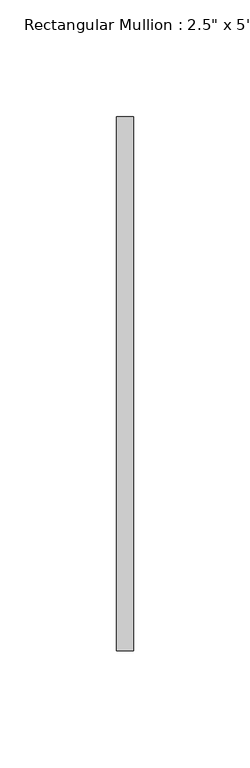
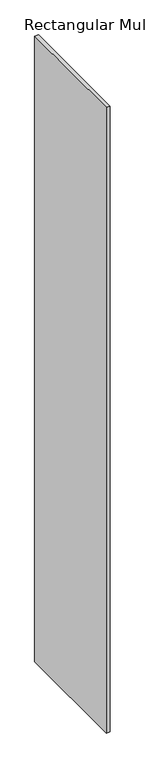
"""IFC4 building model written with IfcOpenShell, lengths in millimetres: member geometry."""

from ifc_helpers import new_model, si_unit, frame, origin, place, context, project, spatial, polyline, outline, extrude, source, transform, mapped, element, save


def member_427a6bf5(model_context):
    return source(origin(), model_context, "Body", "SweptSolid", [
        extrude(outline(polyline([(3.6195, 114.3), (3.6195, -114.3), (-3.6195, -114.3), (-3.6195, 114.3), (3.6195, 114.3)])), frame((0.0, 0.0, -1219.2), z_axis=(0.0, 0.0, 1.0), x_axis=(1.0, 0.0, 0.0)), (0.0, 0.0, 1.0), 1219.2),
    ])


if __name__ == "__main__":
    model = new_model("IFC4")
    model_context = context("Model", 3, world=origin())
    ifc_project = project(units=[si_unit("LENGTHUNIT", "METRE", prefix="MILLI")], contexts=[model_context])
    site = spatial("IfcSite", under=ifc_project)
    building = spatial("IfcBuilding", under=site)
    placement = place(None, origin())
    member_shape = member_427a6bf5(model_context)
    element("IfcMember", 1, ObjectType="Rectangular Mullion : 2.5\" x 5\" rectangular", at=placement, inside=building, context=model_context, shape_type="MappedRepresentation", body=[
        mapped(member_shape, transform((0.0, 0.0, 0.0), x_axis=(1.0, 0.0, 0.0), y_axis=(0.0, 1.0, 0.0), z_axis=(0.0, 0.0, 1.0))),
    ])
    save(model, "model.ifc")

# Revit data of these elements
# Type "Rectangular Mullion : 2.5\" x 5\" rectangular"
#   built-in parameter 1007304 = 0.75 (stored number, unit not read)
#   built-in parameter 1007301 = 0.011875 (stored number, unit not read)
#   built-in parameter 1007300 = 0.011875 (stored number, unit not read)
# Element 1 (IfcMember, "Rectangular Mullion : 2.5\" x 5\" rectangular")
#   Materials on its faces: "WINDOW GLASS MATERIAL"
# Materials
#   "WINDOW GLASS MATERIAL": class "Generic", colour RGB 120 120 120, transparency 0, Cost = 0
